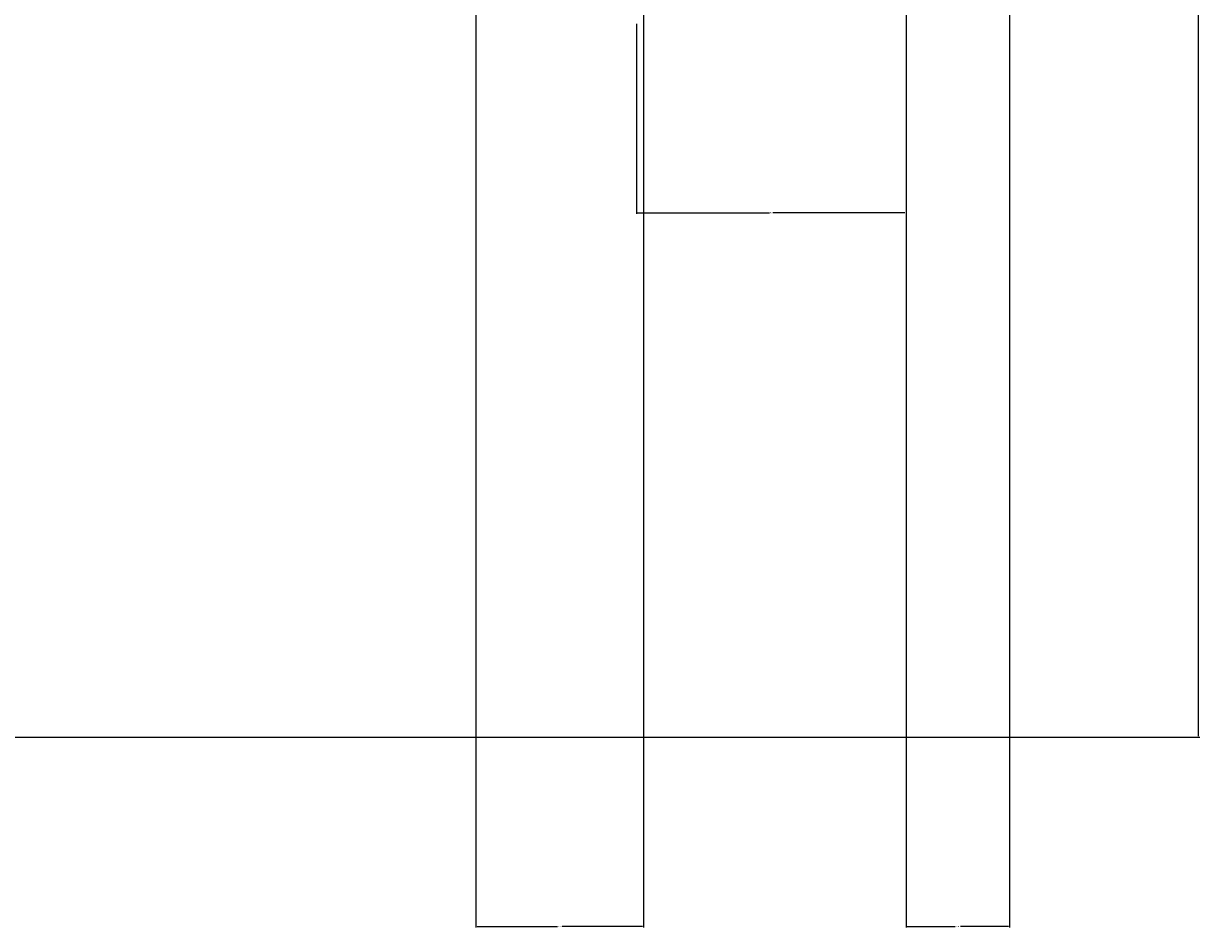
# Model space of a CAD drawing. Units: inches. Extents: x 5 to 421, y -617 to 43.
# Tile 7 of 15: x 223 to 421, y -617 to -465. Entities that reach past the tile are written whole.
import ezdxf

# ---------------------------------------------------------------- set-up
doc = ezdxf.new("R2010")
doc.units = ezdxf.units.IN
doc.header["$MEASUREMENT"] = 0
doc.layers.add('A-ANNO-DIMS', color=2, linetype='Continuous', lineweight=18)
doc.styles.get("Standard").update_dxf_attribs({"font": 'arial.ttf'})
doc.dimstyles.get("Standard").update_dxf_attribs({"dimtxt": 0.18, "dimasz": 0.18, "dimexe": 0.18, "dimexo": 0.0625, "dimgap": 0.09, "dimtad": 0, "dimtih": 1, "dimtoh": 1, "dimdec": 0, "dimzin": 0, "dimdsep": 46, "dimlunit": 3, "dimtxsty": 'Standard', "dimcen": 0.09, "dimadec": 0, "dimazin": 0, "dimtfac": 1, "dimtdec": 0, "dimtofl": 0, "dimtmove": 0, "dimatfit": 3, "dimfxl": 1, "dimtolj": 1, "dimtzin": 0, "dimarcsym": 0})

# ---------------------------------------------------------------- blocks, each defined once
blk = doc.blocks.new('*D55')
at = {"layer": 'A-ANNO-DIMS', "color": 0, "lineweight": -2, "transparency": 16777216}
for p, q in [((370.48, 10.88), (420.4, 10.88)), ((420.22, 10.7), (420.22, -286.69)), ((420.22, -584.44), (420.22, -287.05)), ((169.48, -584.62), (420.4, -584.62))]:
    blk.add_line(p, q, dxfattribs=at)
at = {"layer": 'A-ANNO-DIMS', "color": 0, "transparency": 16777216}
for points in [[(420.19, 10.7), (420.25, 10.7), (420.22, 10.88)], [(420.19, -584.44), (420.25, -584.44), (420.22, -584.62)]]:
    blk.add_solid(points, dxfattribs=at)
at = {"layer": 'Defpoints', "color": 0, "transparency": 16777216}
for p in [(370.42, 10.88), (169.42, -584.62), (420.22, -584.62)]:
    blk.add_point(p, dxfattribs=at)
at = {"layer": 'A-ANNO-DIMS', "color": 0, "transparency": 16777216, "insert": (420.22, -286.87), "char_height": 0.18, "attachment_point": 5}
blk.add_mtext('\\A1;595.5', dxfattribs=at)
blk = doc.blocks.new('*D69')
at = {"layer": 'A-ANNO-DIMS', "color": 0, "lineweight": -2, "transparency": 16777216}
for p, q in [((298.73, -207.41), (298.73, -616.6)), ((326.92, -207.41), (326.92, -616.6)), ((298.91, -616.42), (312.43, -616.42)), ((326.74, -616.42), (313.22, -616.42))]:
    blk.add_line(p, q, dxfattribs=at)
at = {"layer": 'A-ANNO-DIMS', "color": 0, "transparency": 16777216}
for points in [[(298.91, -616.39), (298.91, -616.45), (298.73, -616.42)], [(326.74, -616.39), (326.74, -616.45), (326.92, -616.42)]]:
    blk.add_solid(points, dxfattribs=at)
at = {"layer": 'Defpoints', "color": 0, "transparency": 16777216}
for p in [(298.73, -207.35), (326.92, -207.35), (326.92, -616.42)]:
    blk.add_point(p, dxfattribs=at)
at = {"layer": 'A-ANNO-DIMS', "color": 0, "transparency": 16777216, "insert": (312.82, -616.42), "char_height": 0.18, "attachment_point": 5}
blk.add_mtext('\\A1;28.19', dxfattribs=at)
blk = doc.blocks.new('*D73')
at = {"layer": 'A-ANNO-DIMS', "color": 0, "lineweight": -2, "transparency": 16777216}
for p, q in [((371.03, -247.18), (371.03, -616.6)), ((388.42, -247.18), (388.42, -616.6)), ((371.21, -616.42), (379.27, -616.42)), ((388.24, -616.42), (380.18, -616.42))]:
    blk.add_line(p, q, dxfattribs=at)
at = {"layer": 'A-ANNO-DIMS', "color": 0, "transparency": 16777216}
for points in [[(371.21, -616.39), (371.21, -616.45), (371.03, -616.42)], [(388.24, -616.39), (388.24, -616.45), (388.42, -616.42)]]:
    blk.add_solid(points, dxfattribs=at)
at = {"layer": 'Defpoints', "color": 0, "transparency": 16777216}
for p in [(371.03, -247.12), (388.42, -247.12), (388.42, -616.42)]:
    blk.add_point(p, dxfattribs=at)
at = {"layer": 'A-ANNO-DIMS', "color": 0, "transparency": 16777216, "insert": (379.72, -616.42), "char_height": 0.18, "attachment_point": 5}
blk.add_mtext('\\A1;17.393', dxfattribs=at)
blk = doc.blocks.new('*D75')
at = {"layer": 'A-ANNO-DIMS', "color": 0, "lineweight": -2, "transparency": 16777216}
for p, q in [((325.72, -464.68), (325.72, -496.6)), ((371.03, -464.68), (371.03, -496.6)), ((325.9, -496.42), (348.05, -496.42)), ((370.85, -496.42), (348.7, -496.42))]:
    blk.add_line(p, q, dxfattribs=at)
at = {"layer": 'A-ANNO-DIMS', "color": 0, "transparency": 16777216}
for points in [[(325.9, -496.39), (325.9, -496.45), (325.72, -496.42)], [(370.85, -496.39), (370.85, -496.45), (371.03, -496.42)]]:
    blk.add_solid(points, dxfattribs=at)
at = {"layer": 'Defpoints', "color": 0, "transparency": 16777216}
for p in [(325.72, -464.62), (371.03, -464.62), (325.72, -496.42)]:
    blk.add_point(p, dxfattribs=at)
at = {"layer": 'A-ANNO-DIMS', "color": 0, "transparency": 16777216, "insert": (348.37, -496.42), "char_height": 0.18, "attachment_point": 5}
blk.add_mtext('\\A1;45.3', dxfattribs=at)

msp = doc.modelspace()

# ---------------------------------------------------------------- dimensions: what is measured, and where the dimension line sits
at = {"layer": 'A-ANNO-DIMS'}
for base, p1, p2, angle, picture, middle in [((420.2196, -584.6188), (370.4196, 10.8812), (169.4196, -584.6188), 90, '*D55', (420.2196, -286.8688)), ((325.7231, -496.4188), (371.0265, -464.6188), (325.7231, -464.6188), 180, '*D75', (348.3748, -496.4188))]:
    dim = msp.add_linear_dim(base=base, p1=p1, p2=p2, angle=angle, dimstyle='Standard', override={"dimdec": 1, "dimlfac": 1, "dimrnd": 0, "dimzin": 0, "dimdsep": 46, "dimlunit": 2}, dxfattribs=at)
    dim.commit()
    dim.dimension.update_dxf_attribs({"geometry": picture, "text_midpoint": middle})
for base, p1, p2, override, picture, middle in [((326.9196, -616.4188), (298.7283, -207.3464), (326.9196, -207.3464), {"dimdec": 2, "dimlfac": 1, "dimrnd": 0, "dimzin": 0, "dimdsep": 46, "dimlunit": 2}, '*D69', (312.8239, -616.4188)), ((388.4196, -616.4188), (371.0265, -247.1188), (388.4196, -247.1188), {"dimdec": 3, "dimlfac": 1, "dimrnd": 0, "dimzin": 0, "dimdsep": 46, "dimlunit": 2}, '*D73', (379.7231, -616.4188))]:
    dim = msp.add_linear_dim(base=base, p1=p1, p2=p2, dimstyle='Standard', override=override, dxfattribs=at)
    dim.commit()
    dim.dimension.update_dxf_attribs({"geometry": picture, "text_midpoint": middle})

doc.saveas('drawing.dxf')
